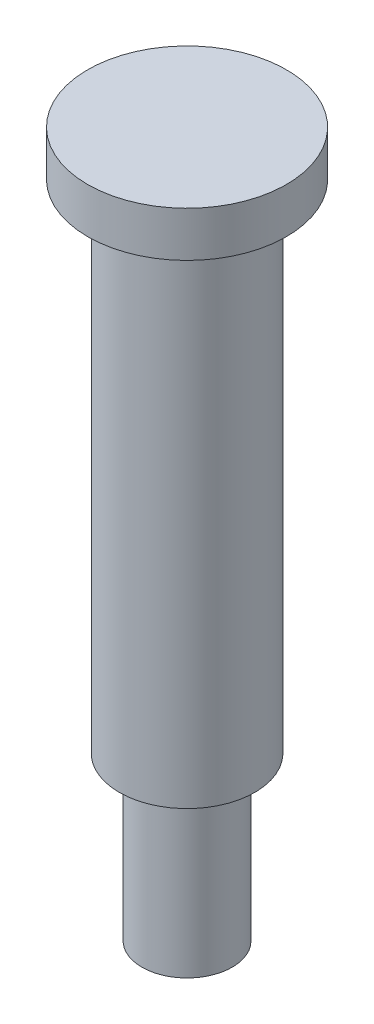
SolidWorks part; units mm, degrees
material "Plain Carbon Steel"
ref_plane "Front Plane" through (0, 0, 0) normal (0, 0, 1) x (1, 0, 0)
ref_plane "Top Plane" through (0, 0, 0) normal (0, 1, 0) x (1, 0, 0)
ref_plane "Right Plane" through (0, 0, 0) normal (1, 0, 0) x (0, 0, -1)
sketch "Pin Profile Sketch" plane through (0, 0, 0) normal (0, 0, 1) x (1, 0, 0)
  line L0 (0, 16.2432) -> (0, -92.2618) construction
  line L1 (0, 0) -> (-11, 0)
  line L2 (-11, 0) -> (-11, -5)
  line L3 (-11, -5) -> (-7.5, -5)
  line L4 (-7.5, -5) -> (-7.5, -60)
  line L5 (-7.5, -60) -> (-5, -60)
  line L6 (-5, -60) -> (-5, -78)
  line L7 (-5, -78) -> (0, -78)
  line L8 (0, 0) -> (0, -78)
  dimension "D1" = 11
  dimension "D2" = 7.5
  dimension "D3" = 5
  dimension "D4" = 5
  dimension "D5" = 78
  dimension "D6" = 18
revolve "Pin Body Revolve" add sketch "Pin Profile Sketch" angle 360 about L0
